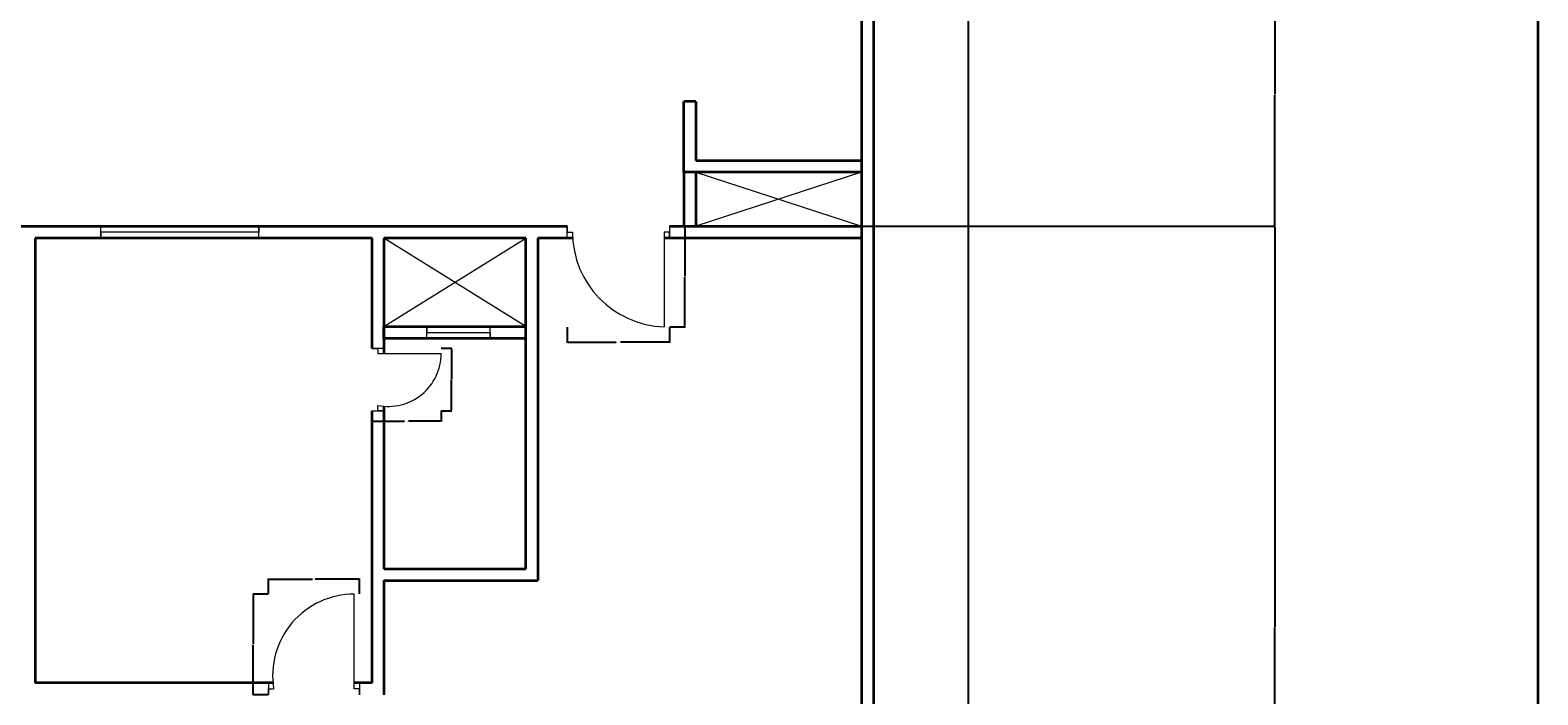
# Model space of a CAD drawing. Units: inches. Extents: x 1520 to 3401, y 1570 to 3432.
# Tile 13 of 15: x 2828 to 3401, y 2061 to 2313. Entities that reach past the tile are written whole.
import ezdxf

# ---------------------------------------------------------------- set-up
doc = ezdxf.new("R2010")
doc.units = ezdxf.units.IN
for name, color, linetype, lineweight in [('A-ANNO-DIMS', 2, 'Continuous', 18), ('A-ANNO-TTLB', 7, 'Continuous', 35), ('A-DOOR', 3, 'Continuous', 18), ('A-FLOR-EDGE', 7, 'Continuous', 25), ('A-FLOR-EVTR', 7, 'Continuous', 35), ('A-FLOR-OPEN', 8, 'Continuous', 13), ('A-GLAZ', 4, 'Continuous', 18), ('A-WALL', 7, 'Continuous', 35)]:
    doc.layers.add(name, color=color, linetype=linetype, lineweight=lineweight)
doc.styles.get("Standard").update_dxf_attribs({"font": 'arial.ttf'})
doc.dimstyles.get("Standard").update_dxf_attribs({"dimtxt": 0.18, "dimasz": 0.18, "dimexe": 0.18, "dimexo": 0.0625, "dimgap": 0.09, "dimtad": 0, "dimtih": 1, "dimtoh": 1, "dimdec": 4, "dimzin": 0, "dimdsep": 46, "dimtxsty": 'Standard', "dimcen": 0.09, "dimadec": 0, "dimazin": 0, "dimtfac": 1, "dimtdec": 4, "dimtofl": 0, "dimtmove": 0, "dimatfit": 3, "dimfxl": 1, "dimtolj": 1, "dimtzin": 0, "dimarcsym": 0})

# ---------------------------------------------------------------- blocks, each defined once
blk = doc.blocks.new('DOOR-SWING-36-16')
for p, q in [((0, 33.75), (0, 38.25)), ((0, 38.25), (0, 36)), ((0, 36), (2, 36)), ((38.88, 36), (36.88, 36)), ((36.88, 36), (36.88, 0)), ((38.88, 38.25), (38.88, 33.75)), ((38.88, 33.75), (38.88, 36)), ((38.88, 36), (38.88, 36))]:
    blk.add_line(p, q)
blk.add_arc((38.02, 36), 36.02, 180, 268.1872)
blk = doc.blocks.new('DOOR-SWING-36-18')
for p, q in [((32.58, 2.25), (32.58, 38.25)), ((0, 4.5), (0, 0)), ((0, 0), (0, 2.25)), ((0, 2.25), (2, 2.25)), ((34.58, 2.25), (32.58, 2.25)), ((34.58, 4.5), (34.58, 0)), ((34.58, 0), (34.58, 2.25))]:
    blk.add_line(p, q)
blk.add_arc((32.58, 7.26), 30.99, 90, 189.3104)
blk = doc.blocks.new('DOOR-SWING-24-19')
for p, q in [((4.5, 23.7), (0, 23.7)), ((0, 23.7), (2.25, 23.7)), ((2.25, 23.7), (2.25, 21.7)), ((2.25, 21.7), (26.25, 21.7)), ((0, 0), (4.5, 0)), ((2.25, 0), (2.25, 2)), ((4.5, 0), (2.25, 0))]:
    blk.add_line(p, q)
blk.add_arc((6.17, 21.7), 20.08, 258.7571, 0)
blk = doc.blocks.new('WIN-PLAN-24-01')
for p, q in [((0, 4.5), (0, 0)), ((0, 0), (0, 2.25)), ((0, 2.25), (24, 2.25)), ((24, 2.25), (24, 4.5)), ((24, 4.5), (24, 0))]:
    blk.add_line(p, q)
blk = doc.blocks.new('WIN-PLAN-60-02')
for p, q in [((4.5, 60), (0, 60)), ((0, 60), (2.25, 60)), ((2.25, 60), (2.25, 0)), ((4.5, 0), (0, 0)), ((2.25, 0), (4.5, 0))]:
    blk.add_line(p, q)
blk = doc.blocks.new('*D111')
at = {"layer": 'A-ANNO-DIMS', "color": 0, "lineweight": -2, "transparency": 16777216}
for p, q in [((3032.07, 2200.37), (3032.07, 2194.42)), ((3070.95, 2200.37), (3070.95, 2194.42)), ((3032.25, 2194.6), (3050.72, 2194.6)), ((3070.77, 2194.6), (3052.3, 2194.6))]:
    blk.add_line(p, q, dxfattribs=at)
at = {"layer": 'A-ANNO-DIMS', "color": 0, "transparency": 16777216}
for points in [[(3032.25, 2194.63), (3032.25, 2194.57), (3032.07, 2194.6)], [(3070.77, 2194.63), (3070.77, 2194.57), (3070.95, 2194.6)]]:
    blk.add_solid(points, dxfattribs=at)
at = {"layer": 'Defpoints', "color": 0, "transparency": 16777216}
for p in [(3032.07, 2200.43), (3070.95, 2200.43), (3070.95, 2194.6)]:
    blk.add_point(p, dxfattribs=at)
at = {"layer": 'A-ANNO-DIMS', "color": 0, "transparency": 16777216, "insert": (3051.51, 2194.6), "char_height": 0.18, "attachment_point": 5}
blk.add_mtext('\\A1;D16 39 TYP.', dxfattribs=at)
blk = doc.blocks.new('*D112')
at = {"layer": 'A-ANNO-DIMS', "color": 0, "lineweight": -2, "transparency": 16777216}
for p, q in [((3071.01, 2238.68), (3076.96, 2238.68)), ((3076.78, 2238.5), (3076.78, 2219.74)), ((3076.78, 2200.61), (3076.78, 2219.37)), ((3071.01, 2200.43), (3076.96, 2200.43))]:
    blk.add_line(p, q, dxfattribs=at)
at = {"layer": 'A-ANNO-DIMS', "color": 0, "transparency": 16777216}
for points in [[(3076.75, 2238.5), (3076.81, 2238.5), (3076.78, 2238.68)], [(3076.75, 2200.61), (3076.81, 2200.61), (3076.78, 2200.43)]]:
    blk.add_solid(points, dxfattribs=at)
at = {"layer": 'Defpoints', "color": 0, "transparency": 16777216}
for p in [(3070.95, 2238.68), (3076.78, 2238.68), (3070.95, 2200.43)]:
    blk.add_point(p, dxfattribs=at)
at = {"layer": 'A-ANNO-DIMS', "color": 0, "transparency": 16777216, "insert": (3076.78, 2219.55), "char_height": 0.18, "attachment_point": 5}
blk.add_mtext('\\A1;38 TYP.', dxfattribs=at)
blk = doc.blocks.new('*D115')
at = {"layer": 'A-ANNO-DIMS', "color": 0, "lineweight": -2, "transparency": 16777216}
for p, q in [((2918.46, 2098.93), (2912.61, 2098.93)), ((2912.79, 2098.75), (2912.79, 2079.99)), ((2912.79, 2060.86), (2912.79, 2079.62)), ((2918.46, 2060.68), (2912.61, 2060.68))]:
    blk.add_line(p, q, dxfattribs=at)
at = {"layer": 'A-ANNO-DIMS', "color": 0, "transparency": 16777216}
for points in [[(2912.76, 2098.75), (2912.82, 2098.75), (2912.79, 2098.93)], [(2912.76, 2060.86), (2912.82, 2060.86), (2912.79, 2060.68)]]:
    blk.add_solid(points, dxfattribs=at)
at = {"layer": 'Defpoints', "color": 0, "transparency": 16777216}
for p in [(2912.79, 2098.93), (2918.52, 2098.93), (2918.52, 2060.68)]:
    blk.add_point(p, dxfattribs=at)
at = {"layer": 'A-ANNO-DIMS', "color": 0, "transparency": 16777216, "insert": (2912.79, 2079.8), "char_height": 0.18, "attachment_point": 5}
blk.add_mtext('\\A1;D18 38 TYP.', dxfattribs=at)
blk = doc.blocks.new('*D116')
at = {"layer": 'A-ANNO-DIMS', "color": 0, "lineweight": -2, "transparency": 16777216}
for p, q in [((2918.52, 2098.99), (2918.52, 2104.85)), ((2918.7, 2104.67), (2935.29, 2104.67)), ((2952.92, 2104.67), (2936.34, 2104.67)), ((2953.1, 2098.99), (2953.1, 2104.85))]:
    blk.add_line(p, q, dxfattribs=at)
at = {"layer": 'A-ANNO-DIMS', "color": 0, "transparency": 16777216}
for points in [[(2918.7, 2104.7), (2918.7, 2104.64), (2918.52, 2104.67)], [(2952.92, 2104.7), (2952.92, 2104.64), (2953.1, 2104.67)]]:
    blk.add_solid(points, dxfattribs=at)
at = {"layer": 'Defpoints', "color": 0, "transparency": 16777216}
for p in [(2953.1, 2104.67), (2918.52, 2098.93), (2953.1, 2098.93)]:
    blk.add_point(p, dxfattribs=at)
at = {"layer": 'A-ANNO-DIMS', "color": 0, "transparency": 16777216, "insert": (2935.81, 2104.67), "char_height": 0.18, "attachment_point": 5}
blk.add_mtext('\\A1;35 TYP.', dxfattribs=at)
blk = doc.blocks.new('*D117')
at = {"layer": 'A-ANNO-DIMS', "color": 0, "lineweight": -2, "transparency": 16777216}
for p, q in [((2957.9, 2168.54), (2957.9, 2164.48)), ((2984.15, 2168.54), (2984.15, 2164.48)), ((2958.08, 2164.66), (2970.23, 2164.66)), ((2983.97, 2164.66), (2971.81, 2164.66))]:
    blk.add_line(p, q, dxfattribs=at)
at = {"layer": 'A-ANNO-DIMS', "color": 0, "transparency": 16777216}
for points in [[(2958.08, 2164.69), (2958.08, 2164.63), (2957.9, 2164.66)], [(2983.97, 2164.69), (2983.97, 2164.63), (2984.15, 2164.66)]]:
    blk.add_solid(points, dxfattribs=at)
at = {"layer": 'Defpoints', "color": 0, "transparency": 16777216}
for p in [(2957.9, 2168.6), (2984.15, 2168.6), (2984.15, 2164.66)]:
    blk.add_point(p, dxfattribs=at)
at = {"layer": 'A-ANNO-DIMS', "color": 0, "transparency": 16777216, "insert": (2971.02, 2164.66), "char_height": 0.18, "attachment_point": 5}
blk.add_mtext('\\A1;D19 26 TYP.', dxfattribs=at)
blk = doc.blocks.new('*D118')
at = {"layer": 'A-ANNO-DIMS', "color": 0, "lineweight": -2, "transparency": 16777216}
for p, q in [((2984.21, 2192.3), (2988.27, 2192.3)), ((2988.09, 2192.12), (2988.09, 2180.63)), ((2988.09, 2168.78), (2988.09, 2180.27)), ((2984.21, 2168.6), (2988.27, 2168.6))]:
    blk.add_line(p, q, dxfattribs=at)
at = {"layer": 'A-ANNO-DIMS', "color": 0, "transparency": 16777216}
for points in [[(2988.06, 2192.12), (2988.12, 2192.12), (2988.09, 2192.3)], [(2988.06, 2168.78), (2988.12, 2168.78), (2988.09, 2168.6)]]:
    blk.add_solid(points, dxfattribs=at)
at = {"layer": 'Defpoints', "color": 0, "transparency": 16777216}
for p in [(2984.15, 2192.3), (2988.09, 2192.3), (2984.15, 2168.6)]:
    blk.add_point(p, dxfattribs=at)
at = {"layer": 'A-ANNO-DIMS', "color": 0, "transparency": 16777216, "insert": (2988.09, 2180.45), "char_height": 0.18, "attachment_point": 5}
blk.add_mtext('\\A1;24 TYP.', dxfattribs=at)
blk = doc.blocks.new('*D196')
at = {"layer": 'A-ANNO-DIMS', "color": 0, "lineweight": -2, "transparency": 16777216}
for p, q in [((3143.96, 2238.68), (3301.09, 2238.68)), ((3300.91, 2238.5), (3300.91, 2086.56)), ((3300.91, 1934.26), (3300.91, 2086.2)), ((3148.46, 1934.08), (3301.09, 1934.08))]:
    blk.add_line(p, q, dxfattribs=at)
at = {"layer": 'A-ANNO-DIMS', "color": 0, "transparency": 16777216}
for points in [[(3300.88, 2238.5), (3300.94, 2238.5), (3300.91, 2238.68)], [(3300.88, 1934.26), (3300.94, 1934.26), (3300.91, 1934.08)]]:
    blk.add_solid(points, dxfattribs=at)
at = {"layer": 'Defpoints', "color": 0, "transparency": 16777216}
for p in [(3143.9, 2238.68), (3300.91, 2238.68), (3148.4, 1934.08)]:
    blk.add_point(p, dxfattribs=at)
at = {"layer": 'A-ANNO-DIMS', "color": 0, "transparency": 16777216, "insert": (3300.91, 2086.38), "char_height": 0.18, "attachment_point": 5}
blk.add_mtext('\\A1;304.6', dxfattribs=at)
blk = doc.blocks.new('*D197')
at = {"layer": 'A-ANNO-DIMS', "color": 0, "lineweight": -2, "transparency": 16777216}
for p, q in [((3143.96, 2338.68), (3301.09, 2338.68)), ((3300.91, 2338.5), (3300.91, 2288.86)), ((3300.91, 2238.86), (3300.91, 2288.5)), ((3143.96, 2238.68), (3301.09, 2238.68))]:
    blk.add_line(p, q, dxfattribs=at)
at = {"layer": 'A-ANNO-DIMS', "color": 0, "transparency": 16777216}
for points in [[(3300.88, 2338.5), (3300.94, 2338.5), (3300.91, 2338.68)], [(3300.88, 2238.86), (3300.94, 2238.86), (3300.91, 2238.68)]]:
    blk.add_solid(points, dxfattribs=at)
at = {"layer": 'Defpoints', "color": 0, "transparency": 16777216}
for p in [(3143.9, 2338.68), (3300.91, 2338.68), (3143.9, 2238.68)]:
    blk.add_point(p, dxfattribs=at)
at = {"layer": 'A-ANNO-DIMS', "color": 0, "transparency": 16777216, "insert": (3300.91, 2288.68), "char_height": 0.18, "attachment_point": 5}
blk.add_mtext('\\A1;100', dxfattribs=at)

msp = doc.modelspace()

# ---------------------------------------------------------------- linework, layer by layer
at = {"layer": 'A-ANNO-TTLB'}
msp.add_lwpolyline([(1519.9253, 3431.7421), (3400.8761, 3431.7421), (3400.8761, 1570.3458), (1519.9253, 1570.3458)], close=True, dxfattribs=at)
at = {"layer": 'A-FLOR-EDGE'}
msp.add_line((3184.3987, 2733.1786), (3184.3987, 1791.6786), dxfattribs=at)
at = {"layer": 'A-FLOR-EVTR'}
for p, q in [((3076.3987, 2259.1786), (3076.3987, 2286.025)), ((3080.8987, 2286.025), (3076.3987, 2286.025)), ((3080.8987, 2286.025), (3080.8987, 2263.6786)), ((3080.8987, 2263.6786), (3143.8987, 2263.6786)), ((3080.8987, 2259.1786), (3076.3987, 2259.1786)), ((3076.3987, 2259.1786), (3076.3987, 2238.6786)), ((3143.8987, 2259.1786), (3080.8987, 2259.1786)), ((3080.8987, 2259.1786), (3080.8987, 2238.6786))]:
    msp.add_line(p, q, dxfattribs=at)
at = {"layer": 'A-FLOR-OPEN'}
for p, q in [((3143.8987, 2259.1786), (3080.8987, 2238.6786)), ((3080.8987, 2259.1786), (3143.8987, 2238.6786)), ((3016.3987, 2200.5887), (2962.3987, 2234.1786)), ((2962.3987, 2200.5887), (3016.3987, 2234.1786))]:
    msp.add_line(p, q, dxfattribs=at)
at = {"layer": 'A-WALL'}
for p, q in [((3143.8987, 2431.1873), (3143.8987, 1963.6868)), ((3148.3987, 2432.7197), (3148.3987, 1965.1342)), ((2819.7132, 2238.6786), (3032.072, 2238.6786)), ((3070.9507, 2238.6786), (3143.8987, 2238.6786)), ((3143.8987, 2238.6786), (3143.8987, 2234.1786)), ((2957.8987, 2234.1786), (2829.8987, 2234.1786)), ((2829.8987, 2234.1786), (2829.8987, 2065.1786)), ((2957.8987, 2192.297), (2957.8987, 2234.1786)), ((3016.3987, 2234.1786), (2962.3987, 2234.1786)), ((2962.3987, 2234.1786), (2962.3987, 2190.297)), ((3016.3987, 2108.5887), (3016.3987, 2234.1786)), ((3034.1424, 2234.1786), (3020.8987, 2234.1786)), ((3020.8987, 2234.1786), (3020.8987, 2104.0887)), ((3143.8987, 2234.1786), (3068.9507, 2234.1786)), ((2962.3987, 2196.0887), (2962.3987, 2200.5887)), ((2962.3987, 2200.5887), (3016.3987, 2200.5887)), ((3016.3987, 2196.0887), (2962.3987, 2196.0887)), ((3016.3987, 2108.5887), (3016.3987, 2196.0887)), ((2957.8987, 2065.1786), (2957.8987, 2168.5982)), ((2962.3987, 2170.282), (2962.3987, 2108.5887)), ((2962.3987, 2108.5887), (3016.3987, 2108.5887)), ((2962.3987, 2104.0887), (2962.3987, 2060.6786)), ((2962.3987, 2104.0887), (3020.8987, 2104.0887)), ((2920.2393, 2065.1786), (2829.8987, 2065.1786)), ((2957.8987, 2065.1786), (2951.1027, 2065.1786))]:
    msp.add_line(p, q, dxfattribs=at)

# ---------------------------------------------------------------- block references
at = {"layer": 'A-DOOR'}
for name, p in [('DOOR-SWING-36-16', (3032.0718, 2200.429)), ('DOOR-SWING-24-19', (2957.8988, 2168.598)), ('DOOR-SWING-36-18', (2918.5238, 2060.679))]:
    msp.add_blockref(name, p, dxfattribs=at)
at = {"layer": 'A-GLAZ', "rotation": 270}
msp.add_blockref('WIN-PLAN-60-02', (2854.9118, 2238.6785), dxfattribs=at)
at = {"layer": 'A-GLAZ', "extrusion": (0, 0, -1), "zscale": -1, "rotation": 180}
msp.add_blockref('WIN-PLAN-24-01', (-2978.7626, 2200.5884), dxfattribs=at)

# ---------------------------------------------------------------- dimensions: what is measured, and where the dimension line sits
at = {"layer": 'A-ANNO-DIMS'}
for base, p1, p2, override, picture, middle in [((3300.9148, 2338.6786), (3143.8987, 2238.6786), (3143.8987, 2338.6786), {"dimdec": 0, "dimlfac": 1, "dimrnd": 0, "dimzin": 0, "dimdsep": 46, "dimlunit": 2}, '*D197', (3300.9148, 2288.6786)), ((3300.9148, 2238.6786), (3148.3987, 1934.0834), (3143.8987, 2238.6786), {"dimdec": 1, "dimlfac": 1, "dimrnd": 0, "dimzin": 0, "dimdsep": 46, "dimlunit": 2}, '*D196', (3300.9148, 2086.381))]:
    dim = msp.add_linear_dim(base=base, p1=p1, p2=p2, angle=90, dimstyle='Standard', override=override, dxfattribs=at)
    dim.commit()
    dim.dimension.update_dxf_attribs({"geometry": picture, "text_midpoint": middle})
for base, p1, p2, text, picture, middle in [((3076.7825, 2238.6786), (3070.9507, 2200.4286), (3070.9507, 2238.6786), '<> TYP.', '*D112', (3076.7825, 2219.5536)), ((2988.0862, 2192.297), (2984.1487, 2168.5982), (2984.1487, 2192.297), '<> TYP.', '*D118', (2988.0862, 2180.4476)), ((2912.7865, 2098.9286), (2918.524, 2060.6786), (2918.524, 2098.9286), 'D18 <> TYP.', '*D115', (2912.7865, 2079.8036))]:
    dim = msp.add_linear_dim(base=base, p1=p1, p2=p2, angle=90, text=text, dimstyle='Standard', override={"dimdec": 0, "dimlfac": 1, "dimrnd": 0, "dimzin": 0, "dimdsep": 46, "dimlunit": 2}, dxfattribs=at)
    dim.commit()
    dim.dimension.update_dxf_attribs({"geometry": picture, "text_midpoint": middle})
for base, p1, p2, text, picture, middle in [((3070.9507, 2194.5968), (3032.072, 2200.4286), (3070.9507, 2200.4286), 'D16 <> TYP.', '*D111', (3051.5114, 2194.5968)), ((2984.1487, 2164.6607), (2957.8987, 2168.5982), (2984.1487, 2168.5982), 'D19 <> TYP.', '*D117', (2971.0237, 2164.6607)), ((2953.1027, 2104.6661), (2918.524, 2098.9286), (2953.1027, 2098.9286), '<> TYP.', '*D116', (2935.8133, 2104.6661))]:
    dim = msp.add_linear_dim(base=base, p1=p1, p2=p2, text=text, dimstyle='Standard', override={"dimdec": 0, "dimlfac": 1, "dimrnd": 0, "dimzin": 0, "dimdsep": 46, "dimlunit": 2}, dxfattribs=at)
    dim.commit()
    dim.dimension.update_dxf_attribs({"geometry": picture, "text_midpoint": middle})

doc.saveas('drawing.dxf')
